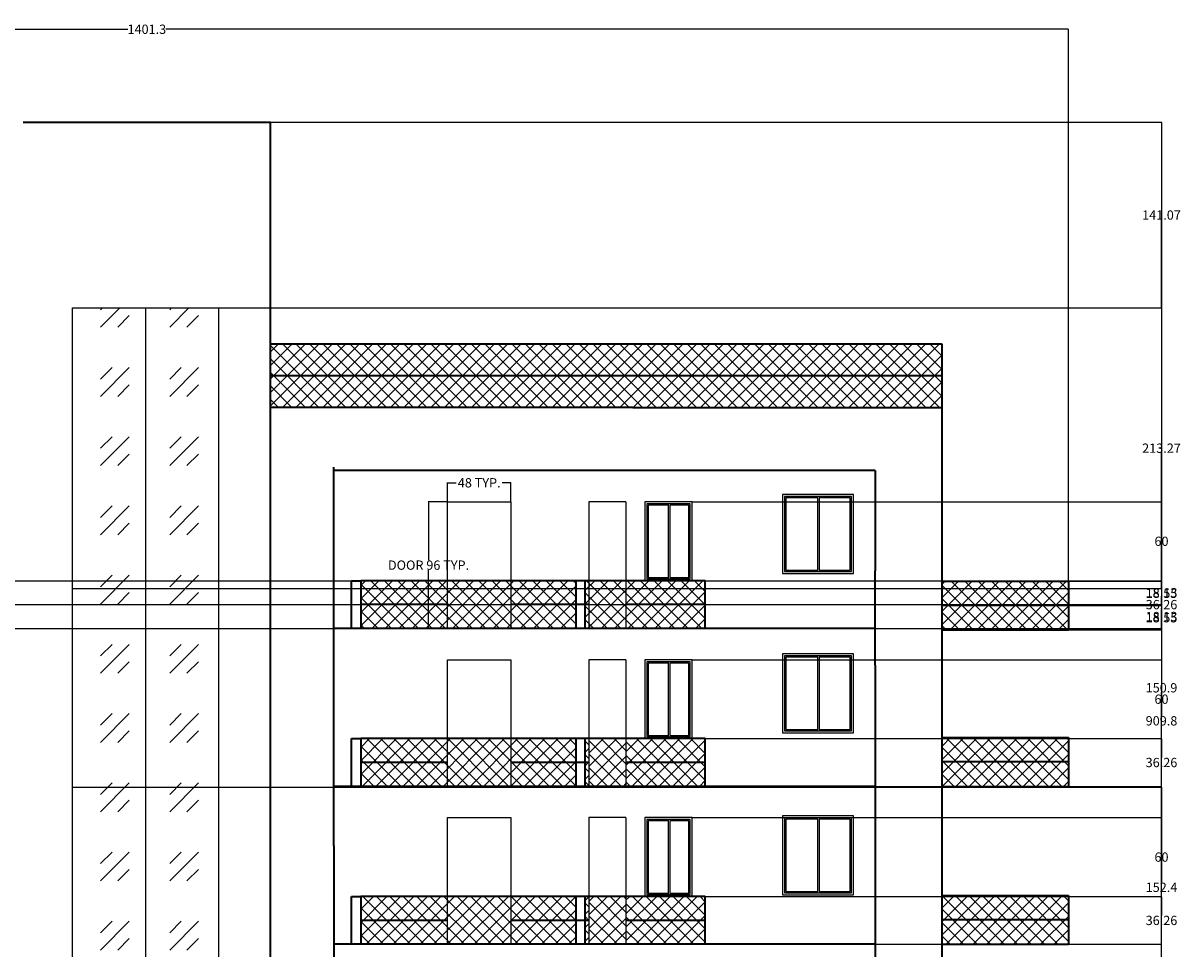
# Model space of a CAD drawing. Units: inches. Extents: x -222 to 1347, y 12 to 1073.
# Tile 4 of 4: x 467 to 1347, y 369 to 1073. Entities that reach past the tile are written whole.
import ezdxf

# ---------------------------------------------------------------- set-up
doc = ezdxf.new("R2010")
doc.units = ezdxf.units.IN
doc.header["$MEASUREMENT"] = 0
for name, color, linetype, lineweight in [('A-ANNO-DIMS', 2, 'Continuous', 18), ('A-DOOR', 4, 'Continuous', 25), ('A-ELEV', 7, 'Continuous', 35), ('A-ELEV-PATT', 8, 'Continuous', 13), ('A-GLAZ', 4, 'Continuous', 25)]:
    doc.layers.add(name, color=color, linetype=linetype, lineweight=lineweight)
doc.styles.get("Standard").update_dxf_attribs({"font": 'arial.ttf'})
doc.dimstyles.get("Standard").update_dxf_attribs({"dimtxt": 7.0625, "dimasz": 0.18, "dimexe": 0.18, "dimexo": 0.0625, "dimgap": 0.09, "dimtad": 0, "dimtih": 1, "dimtoh": 1, "dimdec": 4, "dimzin": 0, "dimdsep": 46, "dimlunit": 4, "dimtxsty": 'Standard', "dimcen": 0.09, "dimadec": 0, "dimazin": 0, "dimtfac": 1, "dimtdec": 4, "dimtofl": 0, "dimtmove": 0, "dimatfit": 3, "dimfxl": 1, "dimtolj": 1, "dimtzin": 0, "dimarcsym": 0})
pattern_1 = [(45, (-188.0434, -1e-13), (-5.126524, 5.126524), []), (135, (-188.0434, -1e-13), (-5.126524, -5.126524), [])]

# ---------------------------------------------------------------- blocks, each defined once
blk = doc.blocks.new('*U2')
for p, q in [((1.5, 1.5), (1.5, 58.5)), ((1.5, 58.5), (27, 58.5)), ((27, 1.5), (27, 58.5)), ((27, 58.5), (52.5, 58.5)), ((52.5, 58.5), (52.5, 1.5)), ((27, 1.5), (1.5, 1.5)), ((52.5, 1.5), (27, 1.5))]:
    blk.add_line(p, q)
blk.add_lwpolyline([(0, 0), (0, 60), (54, 60), (54, 0)], close=True)
for points in [[(26, 57.5), (26, 2.5), (2.5, 2.5), (2.5, 57.5), (26, 57.5)], [(27, 57.5), (51.5, 57.5), (51.5, 2.5), (27, 2.5)]]:
    blk.add_lwpolyline(points)
blk = doc.blocks.new('*U3')
for p, q in [((1.5, 1.5), (1.5, 58.5)), ((1.5, 58.5), (18, 58.5)), ((18, 1.5), (18, 58.5)), ((18, 58.5), (34.5, 58.5)), ((34.5, 58.5), (34.5, 1.5)), ((18, 1.5), (1.5, 1.5)), ((34.5, 1.5), (18, 1.5))]:
    blk.add_line(p, q)
blk.add_lwpolyline([(0, 0), (0, 60), (36, 60), (36, 0)], close=True)
for points in [[(17, 57.5), (17, 2.5), (2.5, 2.5), (2.5, 57.5), (17, 57.5)], [(18, 57.5), (33.5, 57.5), (33.5, 2.5), (18, 2.5)]]:
    blk.add_lwpolyline(points)
blk = doc.blocks.new('DOOR-700')
for p, q in [((0, 96.26), (0, 0)), ((0, 96.26), (23.43, 96.26)), ((23.43, 96.26), (28.14, 96.26)), ((28.14, 96.26), (28.14, 0))]:
    blk.add_line(p, q)
blk = doc.blocks.new('DOOR-1200')
for p, q in [((0, 0), (0, 96.26)), ((0, 96.26), (48.21, 96.26)), ((48.21, 96.26), (48.21, 0))]:
    blk.add_line(p, q)
blk = doc.blocks.new('*D8')
at = {"layer": 'A-ANNO-DIMS', "color": 0, "lineweight": -2, "transparency": 16777216}
for p, q in [((789.85, 709.03), (775.3, 709.03)), ((775.48, 708.85), (775.48, 664.64)), ((775.48, 612.95), (775.48, 657.15)), ((789.85, 612.77), (775.3, 612.77))]:
    blk.add_line(p, q, dxfattribs=at)
at = {"layer": 'A-ANNO-DIMS', "color": 0, "transparency": 16777216}
for points in [[(775.45, 708.85), (775.51, 708.85), (775.48, 709.03)], [(775.45, 612.95), (775.51, 612.95), (775.48, 612.77)]]:
    blk.add_solid(points, dxfattribs=at)
at = {"layer": 'Defpoints', "color": 0, "transparency": 16777216}
for p in [(775.48, 709.03), (789.92, 709.03), (789.92, 612.77)]:
    blk.add_point(p, dxfattribs=at)
at = {"layer": 'A-ANNO-DIMS', "color": 0, "transparency": 16777216, "insert": (775.48, 660.9), "char_height": 7.0625, "attachment_point": 5}
blk.add_mtext('\\A1;DOOR 96 TYP.', dxfattribs=at)
blk = doc.blocks.new('*D9')
at = {"layer": 'A-ANNO-DIMS', "color": 0, "lineweight": -2, "transparency": 16777216}
for p, q in [((789.92, 709.09), (789.92, 723.65)), ((790.1, 723.47), (796.6, 723.47)), ((837.95, 723.47), (831.44, 723.47)), ((838.13, 709.09), (838.13, 723.65))]:
    blk.add_line(p, q, dxfattribs=at)
at = {"layer": 'A-ANNO-DIMS', "color": 0, "transparency": 16777216}
for points in [[(790.1, 723.5), (790.1, 723.44), (789.92, 723.47)], [(837.95, 723.5), (837.95, 723.44), (838.13, 723.47)]]:
    blk.add_solid(points, dxfattribs=at)
at = {"layer": 'Defpoints', "color": 0, "transparency": 16777216}
for p in [(838.13, 723.47), (789.92, 709.03), (838.13, 709.03)]:
    blk.add_point(p, dxfattribs=at)
at = {"layer": 'A-ANNO-DIMS', "color": 0, "transparency": 16777216, "insert": (814.02, 723.47), "char_height": 7.0625, "attachment_point": 5}
blk.add_mtext('\\A1;48 TYP.', dxfattribs=at)
blk = doc.blocks.new('*D10')
at = {"layer": 'A-ANNO-DIMS', "color": 0, "lineweight": -2, "transparency": 16777216}
for p, q in [((-139.29, 648.82), (-139.29, 1068.32)), ((-139.11, 1068.14), (546.95, 1068.14)), ((1261.84, 1068.14), (575.78, 1068.14)), ((1262.02, 648.82), (1262.02, 1068.32))]:
    blk.add_line(p, q, dxfattribs=at)
at = {"layer": 'A-ANNO-DIMS', "color": 0, "transparency": 16777216}
for points in [[(-139.11, 1068.17), (-139.11, 1068.11), (-139.29, 1068.14)], [(1261.84, 1068.17), (1261.84, 1068.11), (1262.02, 1068.14)]]:
    blk.add_solid(points, dxfattribs=at)
at = {"layer": 'Defpoints', "color": 0, "transparency": 16777216}
for p in [(1262.02, 1068.14), (-139.29, 648.76), (1262.02, 648.76)]:
    blk.add_point(p, dxfattribs=at)
at = {"layer": 'A-ANNO-DIMS', "color": 0, "transparency": 16777216, "insert": (561.37, 1068.14), "char_height": 7.062, "attachment_point": 5}
blk.add_mtext('\\A1;1401.3', dxfattribs=at)
blk = doc.blocks.new('*D37')
at = {"layer": 'A-ANNO-DIMS', "color": 0, "lineweight": -2, "transparency": 16777216}
for p, q in [((655.45, 997.49), (1332.85, 997.49)), ((1332.67, 997.31), (1332.67, 546.27)), ((1332.67, 87.84), (1332.67, 538.88)), ((655.45, 87.66), (1332.85, 87.66))]:
    blk.add_line(p, q, dxfattribs=at)
at = {"layer": 'A-ANNO-DIMS', "color": 0, "transparency": 16777216}
for points in [[(1332.64, 997.31), (1332.7, 997.31), (1332.67, 997.49)], [(1332.64, 87.84), (1332.7, 87.84), (1332.67, 87.66)]]:
    blk.add_solid(points, dxfattribs=at)
at = {"layer": 'Defpoints', "color": 0, "transparency": 16777216}
for p in [(655.39, 997.49), (1332.67, 997.49), (655.39, 87.66)]:
    blk.add_point(p, dxfattribs=at)
at = {"layer": 'A-ANNO-DIMS', "color": 0, "transparency": 16777216, "insert": (1332.67, 542.58), "char_height": 7.062, "attachment_point": 5}
blk.add_mtext('\\A1;909.8', dxfattribs=at)
blk = doc.blocks.new('*D58')
at = {"layer": 'A-ANNO-DIMS', "color": 0, "lineweight": -2, "transparency": 16777216}
for p, q in [((1262.08, 630.21), (1332.85, 630.21)), ((1332.67, 630.03), (1332.67, 624.63)), ((1332.67, 611.84), (1332.67, 617.24)), ((1262.08, 611.66), (1332.85, 611.66))]:
    blk.add_line(p, q, dxfattribs=at)
at = {"layer": 'A-ANNO-DIMS', "color": 0, "transparency": 16777216}
for points in [[(1332.64, 630.03), (1332.7, 630.03), (1332.67, 630.21)], [(1332.64, 611.84), (1332.7, 611.84), (1332.67, 611.66)]]:
    blk.add_solid(points, dxfattribs=at)
at = {"layer": 'Defpoints', "color": 0, "transparency": 16777216}
for p in [(1262.02, 630.21), (1332.67, 630.21), (1262.02, 611.66)]:
    blk.add_point(p, dxfattribs=at)
at = {"layer": 'A-ANNO-DIMS', "color": 0, "transparency": 16777216, "insert": (1332.67, 620.93), "char_height": 7.062, "attachment_point": 5}
blk.add_mtext('\\A1;18.55', dxfattribs=at)
blk = doc.blocks.new('*D59')
at = {"layer": 'A-ANNO-DIMS', "color": 0, "lineweight": -2, "transparency": 16777216}
for p, q in [((1262.08, 648.76), (1332.85, 648.76)), ((1332.67, 648.58), (1332.67, 643.18)), ((1332.67, 630.39), (1332.67, 635.79)), ((1262.08, 630.21), (1332.85, 630.21))]:
    blk.add_line(p, q, dxfattribs=at)
at = {"layer": 'A-ANNO-DIMS', "color": 0, "transparency": 16777216}
for points in [[(1332.64, 648.58), (1332.7, 648.58), (1332.67, 648.76)], [(1332.64, 630.39), (1332.7, 630.39), (1332.67, 630.21)]]:
    blk.add_solid(points, dxfattribs=at)
at = {"layer": 'Defpoints', "color": 0, "transparency": 16777216}
for p in [(1262.02, 648.76), (1332.67, 648.76), (1262.02, 630.21)]:
    blk.add_point(p, dxfattribs=at)
at = {"layer": 'A-ANNO-DIMS', "color": 0, "transparency": 16777216, "insert": (1332.67, 639.48), "char_height": 7.062, "attachment_point": 5}
blk.add_mtext('\\A1;18.55', dxfattribs=at)
blk = doc.blocks.new('*D62')
at = {"layer": 'A-ANNO-DIMS', "color": 0, "lineweight": -2, "transparency": 16777216}
for p, q in [((975.9, 409.03), (1332.85, 409.03)), ((1332.67, 408.85), (1332.67, 394.59)), ((1332.67, 372.95), (1332.67, 387.2)), ((985.9, 372.77), (1332.85, 372.77))]:
    blk.add_line(p, q, dxfattribs=at)
at = {"layer": 'A-ANNO-DIMS', "color": 0, "transparency": 16777216}
for points in [[(1332.64, 408.85), (1332.7, 408.85), (1332.67, 409.03)], [(1332.64, 372.95), (1332.7, 372.95), (1332.67, 372.77)]]:
    blk.add_solid(points, dxfattribs=at)
at = {"layer": 'Defpoints', "color": 0, "transparency": 16777216}
for p in [(975.84, 409.03), (1332.67, 409.03), (985.84, 372.77)]:
    blk.add_point(p, dxfattribs=at)
at = {"layer": 'A-ANNO-DIMS', "color": 0, "transparency": 16777216, "insert": (1332.67, 390.9), "char_height": 7.062, "attachment_point": 5}
blk.add_mtext('\\A1;36.26', dxfattribs=at)
blk = doc.blocks.new('*D63')
at = {"layer": 'A-ANNO-DIMS', "color": 0, "lineweight": -2, "transparency": 16777216}
for p, q in [((975.9, 469.03), (1332.85, 469.03)), ((1332.67, 468.85), (1332.67, 442.72)), ((1332.67, 409.21), (1332.67, 435.33)), ((975.9, 409.03), (1332.85, 409.03))]:
    blk.add_line(p, q, dxfattribs=at)
at = {"layer": 'A-ANNO-DIMS', "color": 0, "transparency": 16777216}
for points in [[(1332.64, 468.85), (1332.7, 468.85), (1332.67, 469.03)], [(1332.64, 409.21), (1332.7, 409.21), (1332.67, 409.03)]]:
    blk.add_solid(points, dxfattribs=at)
at = {"layer": 'Defpoints', "color": 0, "transparency": 16777216}
for p in [(975.84, 469.03), (1332.67, 469.03), (975.84, 409.03)]:
    blk.add_point(p, dxfattribs=at)
at = {"layer": 'A-ANNO-DIMS', "color": 0, "transparency": 16777216, "insert": (1332.67, 439.03), "char_height": 7.062, "attachment_point": 5}
blk.add_mtext('\\A1;60', dxfattribs=at)
blk = doc.blocks.new('*D64')
at = {"layer": 'A-ANNO-DIMS', "color": 0, "lineweight": -2, "transparency": 16777216}
for p, q in [((975.9, 529.03), (1332.85, 529.03)), ((1332.67, 528.85), (1332.67, 514.59)), ((1332.67, 492.95), (1332.67, 507.2)), ((985.9, 492.77), (1332.85, 492.77))]:
    blk.add_line(p, q, dxfattribs=at)
at = {"layer": 'A-ANNO-DIMS', "color": 0, "transparency": 16777216}
for points in [[(1332.64, 528.85), (1332.7, 528.85), (1332.67, 529.03)], [(1332.64, 492.95), (1332.7, 492.95), (1332.67, 492.77)]]:
    blk.add_solid(points, dxfattribs=at)
at = {"layer": 'Defpoints', "color": 0, "transparency": 16777216}
for p in [(975.84, 529.03), (1332.67, 529.03), (985.84, 492.77)]:
    blk.add_point(p, dxfattribs=at)
at = {"layer": 'A-ANNO-DIMS', "color": 0, "transparency": 16777216, "insert": (1332.67, 510.9), "char_height": 7.062, "attachment_point": 5}
blk.add_mtext('\\A1;36.26', dxfattribs=at)
blk = doc.blocks.new('*D65')
at = {"layer": 'A-ANNO-DIMS', "color": 0, "lineweight": -2, "transparency": 16777216}
for p, q in [((975.9, 589.03), (1332.85, 589.03)), ((1332.67, 588.85), (1332.67, 562.72)), ((1332.67, 529.21), (1332.67, 555.33)), ((975.9, 529.03), (1332.85, 529.03))]:
    blk.add_line(p, q, dxfattribs=at)
at = {"layer": 'A-ANNO-DIMS', "color": 0, "transparency": 16777216}
for points in [[(1332.64, 588.85), (1332.7, 588.85), (1332.67, 589.03)], [(1332.64, 529.21), (1332.7, 529.21), (1332.67, 529.03)]]:
    blk.add_solid(points, dxfattribs=at)
at = {"layer": 'Defpoints', "color": 0, "transparency": 16777216}
for p in [(975.84, 589.03), (1332.67, 589.03), (975.84, 529.03)]:
    blk.add_point(p, dxfattribs=at)
at = {"layer": 'A-ANNO-DIMS', "color": 0, "transparency": 16777216, "insert": (1332.67, 559.03), "char_height": 7.062, "attachment_point": 5}
blk.add_mtext('\\A1;60', dxfattribs=at)
blk = doc.blocks.new('*D66')
at = {"layer": 'A-ANNO-DIMS', "color": 0, "lineweight": -2, "transparency": 16777216}
for p, q in [((975.9, 649.03), (1332.85, 649.03)), ((1332.67, 648.85), (1332.67, 634.59)), ((1332.67, 612.95), (1332.67, 627.2)), ((985.9, 612.77), (1332.85, 612.77))]:
    blk.add_line(p, q, dxfattribs=at)
at = {"layer": 'A-ANNO-DIMS', "color": 0, "transparency": 16777216}
for points in [[(1332.64, 648.85), (1332.7, 648.85), (1332.67, 649.03)], [(1332.64, 612.95), (1332.7, 612.95), (1332.67, 612.77)]]:
    blk.add_solid(points, dxfattribs=at)
at = {"layer": 'Defpoints', "color": 0, "transparency": 16777216}
for p in [(975.84, 649.03), (1332.67, 649.03), (985.84, 612.77)]:
    blk.add_point(p, dxfattribs=at)
at = {"layer": 'A-ANNO-DIMS', "color": 0, "transparency": 16777216, "insert": (1332.67, 630.9), "char_height": 7.062, "attachment_point": 5}
blk.add_mtext('\\A1;36.26', dxfattribs=at)
blk = doc.blocks.new('*D67')
at = {"layer": 'A-ANNO-DIMS', "color": 0, "lineweight": -2, "transparency": 16777216}
for p, q in [((975.9, 709.03), (1332.85, 709.03)), ((1332.67, 708.85), (1332.67, 682.72)), ((1332.67, 649.21), (1332.67, 675.33)), ((975.9, 649.03), (1332.85, 649.03))]:
    blk.add_line(p, q, dxfattribs=at)
at = {"layer": 'A-ANNO-DIMS', "color": 0, "transparency": 16777216}
for points in [[(1332.64, 708.85), (1332.7, 708.85), (1332.67, 709.03)], [(1332.64, 649.21), (1332.7, 649.21), (1332.67, 649.03)]]:
    blk.add_solid(points, dxfattribs=at)
at = {"layer": 'Defpoints', "color": 0, "transparency": 16777216}
for p in [(975.84, 709.03), (1332.67, 709.03), (975.84, 649.03)]:
    blk.add_point(p, dxfattribs=at)
at = {"layer": 'A-ANNO-DIMS', "color": 0, "transparency": 16777216, "insert": (1332.67, 679.03), "char_height": 7.062, "attachment_point": 5}
blk.add_mtext('\\A1;60', dxfattribs=at)
blk = doc.blocks.new('*D68')
at = {"layer": 'A-ANNO-DIMS', "color": 0, "lineweight": -2, "transparency": 16777216}
for p, q in [((398.84, 630.9), (1332.85, 630.9)), ((1332.67, 630.72), (1332.67, 625.53)), ((1332.67, 612.95), (1332.67, 618.13)), ((405.84, 612.77), (1332.85, 612.77))]:
    blk.add_line(p, q, dxfattribs=at)
at = {"layer": 'A-ANNO-DIMS', "color": 0, "transparency": 16777216}
for points in [[(1332.64, 630.72), (1332.7, 630.72), (1332.67, 630.9)], [(1332.64, 612.95), (1332.7, 612.95), (1332.67, 612.77)]]:
    blk.add_solid(points, dxfattribs=at)
at = {"layer": 'Defpoints', "color": 0, "transparency": 16777216}
for p in [(398.78, 630.9), (1332.67, 630.9), (405.78, 612.77)]:
    blk.add_point(p, dxfattribs=at)
at = {"layer": 'A-ANNO-DIMS', "color": 0, "transparency": 16777216, "insert": (1332.67, 621.83), "char_height": 7.062, "attachment_point": 5}
blk.add_mtext('\\A1;18.13', dxfattribs=at)
blk = doc.blocks.new('*D69')
at = {"layer": 'A-ANNO-DIMS', "color": 0, "lineweight": -2, "transparency": 16777216}
for p, q in [((405.84, 649.03), (1332.85, 649.03)), ((1332.67, 648.85), (1332.67, 643.66)), ((1332.67, 631.08), (1332.67, 636.26)), ((398.84, 630.9), (1332.85, 630.9))]:
    blk.add_line(p, q, dxfattribs=at)
at = {"layer": 'A-ANNO-DIMS', "color": 0, "transparency": 16777216}
for points in [[(1332.64, 648.85), (1332.7, 648.85), (1332.67, 649.03)], [(1332.64, 631.08), (1332.7, 631.08), (1332.67, 630.9)]]:
    blk.add_solid(points, dxfattribs=at)
at = {"layer": 'Defpoints', "color": 0, "transparency": 16777216}
for p in [(405.78, 649.03), (1332.67, 649.03), (398.78, 630.9)]:
    blk.add_point(p, dxfattribs=at)
at = {"layer": 'A-ANNO-DIMS', "color": 0, "transparency": 16777216, "insert": (1332.67, 639.96), "char_height": 7.062, "attachment_point": 5}
blk.add_mtext('\\A1;18.13', dxfattribs=at)
blk = doc.blocks.new('*D72')
at = {"layer": 'A-ANNO-DIMS', "color": 0, "lineweight": -2, "transparency": 16777216}
for p, q in [((615.92, 492.24), (1332.85, 492.24)), ((1332.67, 492.06), (1332.67, 419.74)), ((1332.67, 340.03), (1332.67, 412.35)), ((615.92, 339.85), (1332.85, 339.85))]:
    blk.add_line(p, q, dxfattribs=at)
at = {"layer": 'A-ANNO-DIMS', "color": 0, "transparency": 16777216}
for points in [[(1332.64, 492.06), (1332.7, 492.06), (1332.67, 492.24)], [(1332.64, 340.03), (1332.7, 340.03), (1332.67, 339.85)]]:
    blk.add_solid(points, dxfattribs=at)
at = {"layer": 'Defpoints', "color": 0, "transparency": 16777216}
for p in [(615.85, 492.24), (1332.67, 492.24), (615.85, 339.85)]:
    blk.add_point(p, dxfattribs=at)
at = {"layer": 'A-ANNO-DIMS', "color": 0, "transparency": 16777216, "insert": (1332.67, 416.05), "char_height": 7.062, "attachment_point": 5}
blk.add_mtext('\\A1;152.4', dxfattribs=at)
blk = doc.blocks.new('*D73')
at = {"layer": 'A-ANNO-DIMS', "color": 0, "lineweight": -2, "transparency": 16777216}
for p, q in [((615.92, 643.14), (1332.85, 643.14)), ((1332.67, 642.96), (1332.67, 571.39)), ((1332.67, 492.42), (1332.67, 564)), ((615.92, 492.24), (1332.85, 492.24))]:
    blk.add_line(p, q, dxfattribs=at)
at = {"layer": 'A-ANNO-DIMS', "color": 0, "transparency": 16777216}
for points in [[(1332.64, 642.96), (1332.7, 642.96), (1332.67, 643.14)], [(1332.64, 492.42), (1332.7, 492.42), (1332.67, 492.24)]]:
    blk.add_solid(points, dxfattribs=at)
at = {"layer": 'Defpoints', "color": 0, "transparency": 16777216}
for p in [(615.85, 643.14), (1332.67, 643.14), (615.85, 492.24)]:
    blk.add_point(p, dxfattribs=at)
at = {"layer": 'A-ANNO-DIMS', "color": 0, "transparency": 16777216, "insert": (1332.67, 567.69), "char_height": 7.062, "attachment_point": 5}
blk.add_mtext('\\A1;150.9', dxfattribs=at)
blk = doc.blocks.new('*D74')
at = {"layer": 'A-ANNO-DIMS', "color": 0, "lineweight": -2, "transparency": 16777216}
for p, q in [((615.92, 856.41), (1332.85, 856.41)), ((1332.67, 856.23), (1332.67, 753.48)), ((1332.67, 643.32), (1332.67, 746.08)), ((615.92, 643.14), (1332.85, 643.14))]:
    blk.add_line(p, q, dxfattribs=at)
at = {"layer": 'A-ANNO-DIMS', "color": 0, "transparency": 16777216}
for points in [[(1332.64, 856.23), (1332.7, 856.23), (1332.67, 856.41)], [(1332.64, 643.32), (1332.7, 643.32), (1332.67, 643.14)]]:
    blk.add_solid(points, dxfattribs=at)
at = {"layer": 'Defpoints', "color": 0, "transparency": 16777216}
for p in [(615.85, 856.41), (1332.67, 856.41), (615.85, 643.14)]:
    blk.add_point(p, dxfattribs=at)
at = {"layer": 'A-ANNO-DIMS', "color": 0, "transparency": 16777216, "insert": (1332.67, 749.78), "char_height": 7.062, "attachment_point": 5}
blk.add_mtext('\\A1;213.27', dxfattribs=at)
blk = doc.blocks.new('*D75')
at = {"layer": 'A-ANNO-DIMS', "color": 0, "lineweight": -2, "transparency": 16777216}
for p, q in [((467.41, 997.49), (1332.85, 997.49)), ((1332.67, 997.31), (1332.67, 930.65)), ((1332.67, 856.59), (1332.67, 923.25)), ((615.92, 856.41), (1332.85, 856.41))]:
    blk.add_line(p, q, dxfattribs=at)
at = {"layer": 'A-ANNO-DIMS', "color": 0, "transparency": 16777216}
for points in [[(1332.64, 997.31), (1332.7, 997.31), (1332.67, 997.49)], [(1332.64, 856.59), (1332.7, 856.59), (1332.67, 856.41)]]:
    blk.add_solid(points, dxfattribs=at)
at = {"layer": 'Defpoints', "color": 0, "transparency": 16777216}
for p in [(467.34, 997.49), (1332.67, 997.49), (615.85, 856.41)]:
    blk.add_point(p, dxfattribs=at)
at = {"layer": 'A-ANNO-DIMS', "color": 0, "transparency": 16777216, "insert": (1332.67, 926.95), "char_height": 7.062, "attachment_point": 5}
blk.add_mtext('\\A1;141.07', dxfattribs=at)

msp = doc.modelspace()

# ---------------------------------------------------------------- hatches: boundary and pattern name
at = {"layer": 'A-ELEV-PATT'}
h = msp.add_hatch(dxfattribs=at)
h.set_pattern_fill('GOST_GLASS', color=256, scale=6.2)
h.set_pattern_definition([(45, (0, 0), (52.6087, 0), [31, -43.4]), (45, (13.152, 0), (52.6087, 0), [12.4, -62]), (45, (0, 13.152), (52.6087, 0), [12.4, -62])])
h.paths.add_polyline_path([(560.3092, 856.413), (504.7654, 856.413), (504.7654, 643.1444), (560.3092, 643.1444)])
h.paths.add_polyline_path([(615.8531, 856.413), (560.3092, 856.413), (560.3092, 643.1444), (615.8531, 643.1444)])
h.paths.add_polyline_path([(560.3092, 643.1444), (504.7654, 643.1444), (504.7654, 492.2448), (560.3092, 492.2448)])
h.paths.add_polyline_path([(615.8531, 643.1444), (560.3092, 643.1444), (560.3092, 492.2448), (615.8531, 492.2448)])
h.paths.add_polyline_path([(560.3092, 492.2448), (504.7654, 492.2448), (504.7654, 339.8505), (560.3092, 339.8505)])
h.paths.add_polyline_path([(615.8531, 492.2448), (560.3092, 492.2448), (560.3092, 339.8505), (615.8531, 339.8505)])
h.paths.add_polyline_path([(560.3092, 339.8505), (504.7654, 339.8505), (504.7654, 188.834), (560.3092, 188.834)])
h.paths.add_polyline_path([(615.8531, 339.8505), (560.3092, 339.8505), (560.3092, 188.834), (615.8531, 188.834)])
h = msp.add_hatch(dxfattribs=at)
h.set_pattern_fill('ANSI37', color=256, scale=58)
h.set_pattern_definition(pattern_1)
h.paths.add_polyline_path([(655.387, 828.7653), (1165.8907, 828.7653), (1165.8907, 804.7653), (655.387, 804.7653)])
h.paths.add_polyline_path([(655.387, 804.7653), (1165.8907, 804.7653), (1165.8907, 780.7653), (930.6997, 780.7653), (655.387, 780.7653)])
h = msp.add_hatch(dxfattribs=at)
h.set_pattern_fill('ANSI37', color=256, scale=58)
h.set_pattern_definition(pattern_1)
h.paths.add_polyline_path([(925.5902, 649.0276), (975.8393, 649.0276), (985.8399, 649.0276), (985.8399, 630.8964), (925.5902, 630.8964)])
h.paths.add_polyline_path([(925.5902, 630.8964), (985.8399, 630.8964), (985.8399, 612.7653), (925.5902, 612.7653)])
h.paths.add_polyline_path([(897.4464, 649.0276), (925.5902, 649.0276), (925.5902, 630.8964), (925.5902, 612.7653), (897.4464, 612.7653)])
h.paths.add_polyline_path([(894.63, 649.0276), (897.4464, 649.0276), (897.4464, 630.8964), (894.63, 630.8964)])
h.paths.add_polyline_path([(894.63, 630.8964), (897.4464, 630.8964), (897.4464, 612.7653), (894.63, 612.7653)])
h.paths.add_polyline_path([(838.1288, 649.0276), (887.63, 649.0276), (887.63, 630.8964), (838.1288, 630.8964)])
h.paths.add_polyline_path([(838.1288, 630.8964), (887.63, 630.8964), (887.63, 612.7653), (838.1288, 612.7653)])
h.paths.add_polyline_path([(789.9158, 649.0276), (838.1288, 649.0276), (838.1288, 612.7653), (789.9158, 612.7653)])
h.paths.add_polyline_path([(723.9547, 649.0276), (789.9158, 649.0276), (789.9158, 630.8964), (723.9547, 630.8964)])
h.paths.add_polyline_path([(723.9547, 630.8964), (789.9158, 630.8964), (789.9158, 612.7653), (723.9547, 612.7653)])
h.paths.add_polyline_path([(925.5902, 529.0276), (975.8393, 529.0276), (985.8399, 529.0276), (985.8399, 510.8964), (925.5902, 510.8964)])
h.paths.add_polyline_path([(925.5902, 510.8964), (985.8399, 510.8964), (985.8399, 492.7653), (925.5902, 492.7653)])
h.paths.add_polyline_path([(894.63, 529.0276), (897.4464, 529.0276), (897.4464, 510.9211), (894.63, 510.9211)])
h.paths.add_polyline_path([(894.63, 510.9211), (897.4464, 510.9211), (897.4464, 492.7653), (894.63, 492.7653)])
h.paths.add_polyline_path([(838.1288, 529.0276), (887.63, 529.0276), (887.63, 510.9211), (838.1288, 510.9211)])
h.paths.add_polyline_path([(838.1288, 510.9211), (887.63, 510.9211), (887.63, 492.7653), (838.1288, 492.7653)])
h.paths.add_polyline_path([(789.9158, 529.0276), (838.1288, 529.0276), (838.1288, 510.9211), (838.1288, 492.7653), (789.9158, 492.7653)])
h.paths.add_polyline_path([(723.9547, 529.0276), (789.9158, 529.0276), (789.9158, 510.9211), (723.9547, 510.9211)])
h.paths.add_polyline_path([(723.9547, 510.9211), (789.9158, 510.9211), (789.9158, 492.7653), (723.9547, 492.7653)])
h.paths.add_polyline_path([(723.9547, 409.0276), (789.9158, 409.0276), (789.9158, 390.8964), (723.9547, 390.8964)])
h.paths.add_polyline_path([(723.9547, 390.8964), (789.9158, 390.8964), (789.9158, 372.7653), (723.9547, 372.7653)])
h.paths.add_polyline_path([(838.1288, 409.0276), (887.63, 409.0276), (887.63, 390.8964), (838.1288, 390.8964)])
h.paths.add_polyline_path([(789.9158, 409.0276), (838.1288, 409.0276), (838.1288, 390.8964), (838.1288, 372.7653), (789.9158, 372.7653), (789.9158, 390.8964)])
h.paths.add_polyline_path([(838.1288, 390.8964), (887.63, 390.8964), (887.63, 372.7653), (838.1288, 372.7653)])
h.paths.add_polyline_path([(894.63, 409.0276), (897.4464, 409.0276), (897.4464, 390.8964), (894.63, 390.8964)])
h.paths.add_polyline_path([(894.63, 390.8964), (897.4464, 390.8964), (897.4464, 372.7653), (894.63, 372.7653)])
h.paths.add_polyline_path([(925.5902, 409.0276), (975.8393, 409.0276), (985.8399, 409.0276), (985.8399, 390.8964), (925.5902, 390.8964)])
h.paths.add_polyline_path([(925.5902, 390.8964), (985.8399, 390.8964), (985.8399, 372.7653), (925.5902, 372.7653)])
h = msp.add_hatch(dxfattribs=at)
h.set_pattern_fill('ANSI37', color=256, scale=58)
h.set_pattern_definition(pattern_1)
h.paths.add_polyline_path([(1165.8907, 648.7576), (1262.0222, 648.7576), (1262.0222, 630.2077), (1165.8907, 630.2077)])
h.paths.add_polyline_path([(1165.8907, 630.2077), (1262.0222, 630.2077), (1262.0222, 611.6578), (1165.8907, 611.6578)])
h.paths.add_polyline_path([(1165.8907, 529.8651), (1262.0222, 529.8651), (1262.0222, 511.3152), (1165.8907, 511.3152)])
h.paths.add_polyline_path([(1165.8907, 511.3152), (1262.0222, 511.3152), (1262.0222, 492.7653), (1165.8907, 492.7653)])
h.paths.add_polyline_path([(1165.8907, 409.8651), (1262.0222, 409.8651), (1262.0222, 391.3152), (1165.8907, 391.3152)])
h.paths.add_polyline_path([(1165.8907, 391.3152), (1262.0222, 391.3152), (1262.0222, 372.7653), (1165.8907, 372.7653)])
h.paths.add_polyline_path([(1165.8907, 244.764), (1262.0222, 244.764), (1262.0222, 226.2141), (1165.8907, 226.2141)])
h.paths.add_polyline_path([(1165.8907, 226.2141), (1262.0222, 226.2141), (1262.0222, 207.6642), (1165.8907, 207.6642)])
h = msp.add_hatch(dxfattribs=at)
h.set_pattern_fill('ANSI37', color=256, scale=58)
h.paths.add_polyline_path([(925.5902, 529.0276), (897.4464, 529.0276), (897.4464, 492.7653), (925.5902, 492.7653)])
h.paths.add_polyline_path([(925.5902, 409.0276), (897.4464, 409.0276), (897.4464, 372.7653), (925.5902, 372.7653)])
h.paths.add_polyline_path([(225.2842, 409.0276), (197.1405, 409.0276), (197.1405, 372.7653), (225.2842, 372.7653)])
h.paths.add_polyline_path([(225.2842, 529.0276), (197.1405, 529.0276), (197.1405, 492.7653), (225.2842, 492.7653)])

# ---------------------------------------------------------------- linework, layer by layer
at = {"layer": 'A-ELEV'}
for p, q in [((467.3436, 997.488), (655.387, 997.488)), ((655.387, 87.6642), (655.387, 997.488)), ((1165.8907, 828.7653), (655.387, 828.7653)), ((1165.8907, 780.7653), (1165.8907, 828.7653)), ((1165.8907, 804.7653), (655.387, 804.7653)), ((930.6997, 780.7653), (655.387, 780.7653)), ((930.6997, 780.7653), (1165.8907, 780.7653)), ((1165.8907, 207.6642), (1165.8907, 780.7653)), ((703.387, 447.6642), (703.387, 735.4477)), ((1114.924, 732.7653), (703.387, 732.7653)), ((1114.924, 732.7653), (1114.924, 656.5028)), ((1114.924, 584.7569), (1114.924, 656.5028)), ((716.9547, 612.7653), (716.9547, 649.0276)), ((716.9547, 649.0276), (723.9547, 649.0276)), ((975.8393, 649.0276), (723.9547, 649.0276)), ((723.9547, 649.0276), (723.9547, 612.7653)), ((887.63, 612.7653), (887.63, 649.0276)), ((894.63, 612.7653), (894.63, 649.0276)), ((985.8399, 649.0276), (975.8393, 649.0276)), ((985.8399, 612.7653), (985.8399, 649.0276)), ((1165.8907, 648.7576), (1262.0222, 648.7576)), ((1262.0222, 648.7576), (1262.0222, 611.6578)), ((789.9158, 630.8964), (723.9547, 630.8964)), ((897.4464, 630.8964), (838.1288, 630.8964)), ((985.8399, 630.8964), (925.5902, 630.8964)), ((1262.0222, 630.2077), (1165.8907, 630.2077)), ((1114.924, 612.7653), (703.387, 612.7653)), ((1165.8907, 611.6578), (1262.0222, 611.6578)), ((1114.924, 584.7569), (1114.924, 347.9663)), ((716.9547, 492.7653), (716.9547, 529.0276)), ((716.9547, 529.0276), (723.9547, 529.0276)), ((975.8393, 529.0276), (723.9547, 529.0276)), ((723.9547, 529.0276), (723.9547, 492.7653)), ((887.63, 492.7653), (887.63, 529.0276)), ((894.63, 492.7653), (894.63, 529.0276)), ((985.8399, 529.0276), (975.8393, 529.0276)), ((985.8399, 492.7653), (985.8399, 529.0276)), ((1165.8907, 529.8651), (1262.0222, 529.8651)), ((1262.0222, 529.8651), (1262.0222, 492.7653)), ((789.9158, 510.9211), (723.9547, 510.9211)), ((897.4464, 510.9211), (838.1288, 510.9211)), ((985.8399, 510.8964), (925.5902, 510.8964)), ((1262.0222, 511.3152), (1165.8907, 511.3152)), ((1114.924, 492.7653), (703.387, 492.7653)), ((1165.8907, 492.7653), (1262.0222, 492.7653)), ((703.387, 447.6642), (703.387, 327.6642)), ((716.9547, 372.7653), (716.9547, 409.0276)), ((716.9547, 409.0276), (723.9547, 409.0276)), ((975.8393, 409.0276), (723.9547, 409.0276)), ((723.9547, 409.0276), (723.9547, 372.7653)), ((887.63, 372.7653), (887.63, 409.0276)), ((894.63, 372.7653), (894.63, 409.0276)), ((985.8399, 409.0276), (975.8393, 409.0276)), ((985.8399, 372.7653), (985.8399, 409.0276)), ((1165.8907, 409.8651), (1262.0222, 409.8651)), ((1262.0222, 409.8651), (1262.0222, 372.7653)), ((789.9158, 390.8964), (723.9547, 390.8964)), ((897.4464, 390.8964), (838.1288, 390.8964)), ((985.8399, 390.8964), (925.5902, 390.8964)), ((1262.0222, 391.3152), (1165.8907, 391.3152)), ((1114.924, 372.7653), (703.387, 372.7653)), ((1165.8907, 372.7653), (1262.0222, 372.7653))]:
    msp.add_line(p, q, dxfattribs=at)
at = {"layer": 'A-GLAZ'}
for p, q in [((560.3092, 856.413), (560.3092, 188.834)), ((504.7654, 643.1444), (615.8531, 643.1444)), ((504.7654, 492.2448), (615.8531, 492.2448))]:
    msp.add_line(p, q, dxfattribs=at)
msp.add_lwpolyline([(504.7654, 856.413), (615.8531, 856.413), (615.8531, 188.834), (504.7654, 188.834)], close=True, dxfattribs=at)

# ---------------------------------------------------------------- block references
at = {"layer": 'A-DOOR'}
for p in [(789.9161, 612.7651), (789.9161, 492.7651), (789.9161, 372.7651)]:
    msp.add_blockref('DOOR-1200', p, dxfattribs=at)
at = {"layer": 'A-DOOR', "extrusion": (0, 0, -1), "zscale": -1}
for p in [(-925.5906, 612.7651), (-925.5906, 492.7651), (-925.5906, 372.7651)]:
    msp.add_blockref('DOOR-700', p, dxfattribs=at)
at = {"layer": 'A-GLAZ', "xscale": -1}
for name, p in [('*U2', (1098.5315, 654.4958)), ('*U3', (975.8393, 649.0276)), ('*U2', (1098.5315, 533.4746)), ('*U3', (975.8393, 529.0276)), ('*U3', (975.8393, 409.0276)), ('*U2', (1098.5315, 410.3378))]:
    msp.add_blockref(name, p, dxfattribs=at)

# ---------------------------------------------------------------- dimensions: what is measured, and where the dimension line sits
at = {"layer": 'A-ANNO-DIMS'}
dim = msp.add_linear_dim(base=(1262.0222, 1068.138), p1=(-139.2916, 648.7576), p2=(1262.0222, 648.7576), dimstyle='Standard', override={"dimdec": 1, "dimlfac": 1, "dimrnd": 0, "dimzin": 0, "dimdsep": 46, "dimlunit": 2}, dxfattribs=at)
dim.commit()
dim.dimension.update_dxf_attribs({"geometry": '*D10', "text_midpoint": (561.3653, 1068.138)})
for base, p1, p2, override, picture, middle in [((1332.67221, 997.48798), (615.85307, 856.41299), (467.34363, 997.48798), {"dimdec": 2, "dimlfac": 1, "dimrnd": 0, "dimzin": 0, "dimdsep": 46, "dimlunit": 2}, '*D75', (1332.67221, 926.95048)), ((1332.6722, 997.488), (655.387, 87.6642), (655.387, 997.488), {"dimdec": 1, "dimlfac": 1, "dimrnd": 0, "dimzin": 0, "dimdsep": 46, "dimlunit": 2}, '*D37', (1332.6722, 542.5761)), ((1332.6722, 856.413), (615.8531, 643.1444), (615.8531, 856.413), {"dimdec": 2, "dimlfac": 1, "dimrnd": 0, "dimzin": 0, "dimdsep": 46, "dimlunit": 2}, '*D74', (1332.6722, 749.7787)), ((1332.6722, 709.0276), (975.8393, 649.0276), (975.8393, 709.0276), {"dimdec": 0, "dimlfac": 1, "dimrnd": 0, "dimzin": 0, "dimdsep": 46, "dimlunit": 2}, '*D67', (1332.6722, 679.0276)), ((1332.6722, 649.0276), (398.776, 630.8964), (405.776, 649.0276), {"dimdec": 2, "dimlfac": 1, "dimrnd": 0, "dimzin": 0, "dimdsep": 46, "dimlunit": 2}, '*D69', (1332.6722, 639.962)), ((1332.6722, 643.1444), (615.8531, 492.2448), (615.8531, 643.1444), {"dimdec": 1, "dimlfac": 1, "dimrnd": 0, "dimzin": 0, "dimdsep": 46, "dimlunit": 2}, '*D73', (1332.6722, 567.6946)), ((1332.6722, 649.0276), (985.8399, 612.7653), (975.8393, 649.0276), {"dimdec": 2, "dimlfac": 1, "dimrnd": 0, "dimzin": 0, "dimdsep": 46, "dimlunit": 2}, '*D66', (1332.6722, 630.8964)), ((1332.6722, 648.7576), (1262.0222, 630.2077), (1262.0222, 648.7576), {"dimdec": 2, "dimlfac": 1, "dimrnd": 0, "dimzin": 0, "dimdsep": 46, "dimlunit": 2}, '*D59', (1332.6722, 639.4827)), ((1332.6722, 630.8964), (405.776, 612.7653), (398.776, 630.8964), {"dimdec": 2, "dimlfac": 1, "dimrnd": 0, "dimzin": 0, "dimdsep": 46, "dimlunit": 2}, '*D68', (1332.6722, 621.8309)), ((1332.6722, 630.2077), (1262.0222, 611.6578), (1262.0222, 630.2077), {"dimdec": 2, "dimlfac": 1, "dimrnd": 0, "dimzin": 0, "dimdsep": 46, "dimlunit": 2}, '*D58', (1332.6722, 620.9328)), ((1332.6722, 589.0276), (975.8393, 529.0276), (975.8393, 589.0276), {"dimdec": 0, "dimlfac": 1, "dimrnd": 0, "dimzin": 0, "dimdsep": 46, "dimlunit": 2}, '*D65', (1332.6722, 559.0276)), ((1332.6722, 529.0276), (985.8399, 492.7653), (975.8393, 529.0276), {"dimdec": 2, "dimlfac": 1, "dimrnd": 0, "dimzin": 0, "dimdsep": 46, "dimlunit": 2}, '*D64', (1332.6722, 510.8964)), ((1332.6722, 492.2448), (615.8531, 339.8505), (615.8531, 492.2448), {"dimdec": 1, "dimlfac": 1, "dimrnd": 0, "dimzin": 0, "dimdsep": 46, "dimlunit": 2}, '*D72', (1332.6722, 416.0477)), ((1332.6722, 469.0276), (975.8393, 409.0276), (975.8393, 469.0276), {"dimdec": 0, "dimlfac": 1, "dimrnd": 0, "dimzin": 0, "dimdsep": 46, "dimlunit": 2}, '*D63', (1332.6722, 439.0276)), ((1332.6722, 409.0276), (985.8399, 372.7653), (975.8393, 409.0276), {"dimdec": 2, "dimlfac": 1, "dimrnd": 0, "dimzin": 0, "dimdsep": 46, "dimlunit": 2}, '*D62', (1332.6722, 390.8964))]:
    dim = msp.add_linear_dim(base=base, p1=p1, p2=p2, angle=90, dimstyle='Standard', override=override, dxfattribs=at)
    dim.commit()
    dim.dimension.update_dxf_attribs({"geometry": picture, "text_midpoint": middle})
dim = msp.add_linear_dim(base=(838.1288, 723.4669), p1=(789.9158, 709.0276), p2=(838.1288, 709.0276), text='<> TYP.', dimstyle='Standard', override={"dimdec": 0, "dimlfac": 1, "dimrnd": 0, "dimzin": 0, "dimdsep": 46, "dimlunit": 2}, dxfattribs=at)
dim.commit()
dim.dimension.update_dxf_attribs({"geometry": '*D9', "text_midpoint": (814.0223, 723.4669)})
dim = msp.add_linear_dim(base=(775.4765, 709.0276), p1=(789.9158, 612.7653), p2=(789.9158, 709.0276), angle=90, text='DOOR <> TYP.', dimstyle='Standard', override={"dimdec": 0, "dimlfac": 1, "dimrnd": 0, "dimzin": 0, "dimdsep": 46, "dimlunit": 2}, dxfattribs=at)
dim.commit()
dim.dimension.update_dxf_attribs({"geometry": '*D8', "text_midpoint": (775.4765, 660.8964)})

doc.saveas('drawing.dxf')
